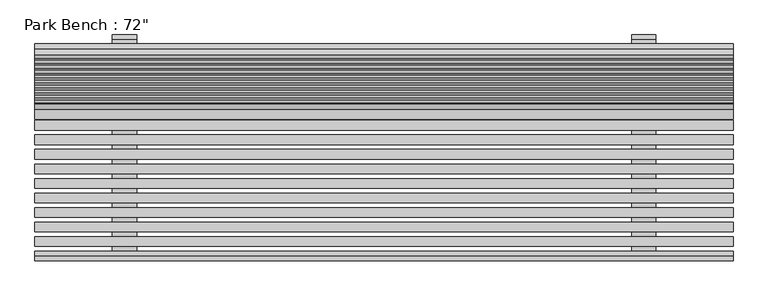
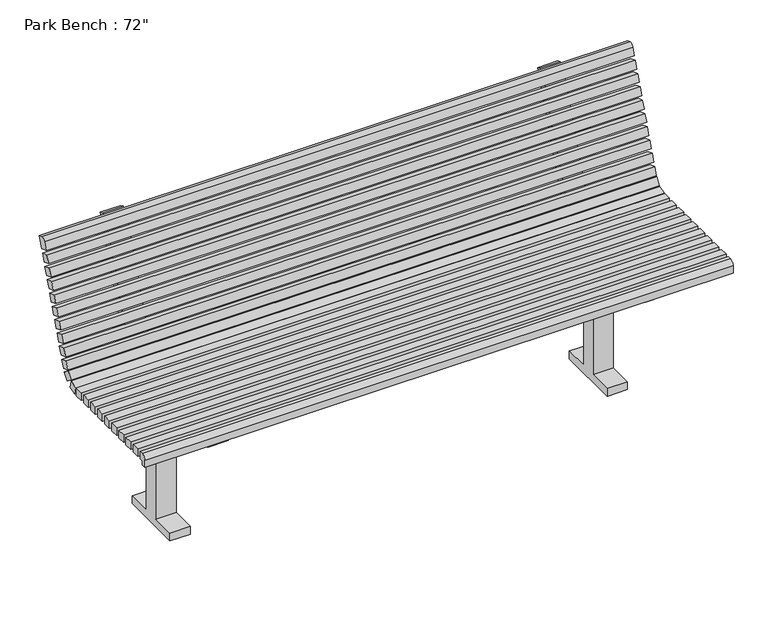
"""IFC4 building model written with IfcOpenShell, lengths in millimetres: geographic element geometry."""

from ifc_helpers import new_model, si_unit, point, frame, frame_2d, origin, place, context, project, spatial, polyline, circle_curve, trimmed, segment, composite_curve, outline, extrude, source, transform, mapped, element, save


def geographic_element_235d1464(model_context):
    return source(origin(), model_context, "Body", "SweptSolid", [
        extrude(outline(polyline([(914.4, -255.4337104), (914.4, -280.8337104), (-914.4, -280.8337104), (-914.4, -255.4337104), (914.4, -255.4337104)])), frame((0.0, 0.0, 457.2), z_axis=(0.0, 0.0, 1.0), x_axis=(1.0, 0.0, 0.0)), (0.0, 0.0, 1.0), 25.4),
        extrude(outline(polyline([(914.4, -217.3337104), (914.4, -242.7337104), (-914.4, -242.7337104), (-914.4, -217.3337104), (914.4, -217.3337104)])), frame((0.0, 0.0, 457.2), z_axis=(0.0, 0.0, 1.0), x_axis=(1.0, 0.0, 0.0)), (0.0, 0.0, 1.0), 25.4),
        extrude(outline(polyline([(914.4, -179.2337104), (914.4, -204.6337104), (-914.4, -204.6337104), (-914.4, -179.2337104), (914.4, -179.2337104)])), frame((0.0, 0.0, 457.2), z_axis=(0.0, 0.0, 1.0), x_axis=(1.0, 0.0, 0.0)), (0.0, 0.0, 1.0), 25.4),
        extrude(outline(polyline([(914.4, -141.1337104), (914.4, -166.5337104), (-914.4, -166.5337104), (-914.4, -141.1337104), (914.4, -141.1337104)])), frame((0.0, 0.0, 457.2), z_axis=(0.0, 0.0, 1.0), x_axis=(1.0, 0.0, 0.0)), (0.0, 0.0, 1.0), 25.4),
        extrude(outline(polyline([(914.4, -103.0337104), (914.4, -128.4337104), (-914.4, -128.4337104), (-914.4, -103.0337104), (914.4, -103.0337104)])), frame((0.0, 0.0, 457.2), z_axis=(0.0, 0.0, 1.0), x_axis=(1.0, 0.0, 0.0)), (0.0, 0.0, 1.0), 25.4),
        extrude(outline(polyline([(914.4, -64.9337104), (914.4, -90.3337104), (-914.4, -90.3337104), (-914.4, -64.9337104), (914.4, -64.9337104)])), frame((0.0, 0.0, 457.2), z_axis=(0.0, 0.0, 1.0), x_axis=(1.0, 0.0, 0.0)), (0.0, 0.0, 1.0), 25.4),
        extrude(outline(polyline([(914.4, -26.8337104), (914.4, -52.2337104), (-914.4, -52.2337104), (-914.4, -26.8337104), (914.4, -26.8337104)])), frame((0.0, 0.0, 457.2), z_axis=(0.0, 0.0, 1.0), x_axis=(1.0, 0.0, 0.0)), (0.0, 0.0, 1.0), 25.4),
        extrude(outline(polyline([(914.4, 11.2662896), (914.4, -14.1337104), (-914.4, -14.1337104), (-914.4, 11.2662896), (914.4, 11.2662896)])), frame((0.0, 0.0, 457.2), z_axis=(0.0, 0.0, 1.0), x_axis=(1.0, 0.0, 0.0)), (0.0, 0.0, 1.0), 25.4),
        extrude(outline(polyline([(914.4, 49.3662896), (914.4, 23.9662896), (-914.4, 23.9662896), (-914.4, 49.3662896), (914.4, 49.3662896)])), frame((0.0, 0.0, 457.2), z_axis=(0.0, 0.0, 1.0), x_axis=(1.0, 0.0, 0.0)), (0.0, 0.0, 1.0), 25.4),
        extrude(outline(composite_curve([segment(polyline([(-304.8, 457.2), (-304.8, 444.5), (-318.9337104, 444.5), (-318.9337104, 468.3125)]), True, "CONTINUOUS"), segment(trimmed(circle_curve(frame_2d((-304.6462104, 468.3125)), 14.2875), [point((-318.9337104, 468.3125))], [point((-304.6462104, 482.6))], False, "CARTESIAN"), True, "CONTINUOUS"), segment(polyline([(-304.6462104, 482.6), (-293.5337104, 482.6), (-293.5337104, 457.2), (-304.8, 457.2)]), True, "CONTINUOUS")], self_intersect=False)), frame((-914.4, 0.0, 0.0), z_axis=(1.0, 0.0, 0.0), x_axis=(0.0, 1.0, 0.0)), (0.0, 0.0, 1.0), 1828.8),
        extrude(outline(polyline([(0.0, -25.4), (0.0, 0.0), (1828.8, 0.0), (1828.8, -25.4), (0.0, -25.4)])), frame((914.4, 121.2738625, 585.5181247), z_axis=(0.0, 0.342020143325687, 0.9396926207859018), x_axis=(-1.0, 0.0, 0.0)), (0.0, 0.0, 1.0), 25.4),
        extrude(outline(polyline([(0.0, -25.4), (0.0, 0.0), (1828.8, 0.0), (1828.8, -25.4), (0.0, -25.4)])), frame((914.4, 134.30483, 621.3204136), z_axis=(0.0, 0.34202014332568254, 0.9396926207859034), x_axis=(-1.0, 0.0, 0.0)), (0.0, 0.0, 1.0), 25.4),
        extrude(outline(polyline([(0.0, -25.3999999), (0.0, 0.0), (1828.8, 0.0), (1828.8, -25.3999999), (0.0, -25.3999999)])), frame((914.4, 95.2119276, 513.913547), z_axis=(0.0, 0.34202014332568254, 0.9396926207859034), x_axis=(-1.0, 0.0, 0.0)), (0.0, 0.0, 1.0), 25.4),
        extrude(outline(polyline([(0.0, -25.4000001), (0.0, 0.0), (1828.8, 0.0), (1828.8, -25.4000001), (0.0, -25.4000001)])), frame((914.4, 108.242895, 549.7158359), z_axis=(0.0, 0.34202014332567804, 0.9396926207859051), x_axis=(-1.0, 0.0, 0.0)), (0.0, 0.0, 1.0), 25.4),
        extrude(outline(polyline([(0.0, -25.4), (0.0, 0.0), (1828.8, 0.0), (1828.8, -25.4), (0.0, -25.4)])), frame((914.4, 173.3977323, 728.7272801), z_axis=(0.0, 0.34202014332568337, 0.9396926207859031), x_axis=(-1.0, 0.0, 0.0)), (0.0, 0.0, 1.0), 25.4),
        extrude(outline(polyline([(0.0, -25.4000001), (0.0, 0.0), (1828.8, 0.0), (1828.8, -25.4000001), (0.0, -25.4000001)])), frame((914.4, 186.4286998, 764.529569), z_axis=(0.0, 0.3420201433256829, 0.9396926207859032), x_axis=(-1.0, 0.0, 0.0)), (0.0, 0.0, 1.0), 25.4),
        extrude(outline(polyline([(0.0, -25.4), (0.0, 0.0), (1828.8, 0.0), (1828.8, -25.4), (0.0, -25.4)])), frame((914.4, 147.3357974, 657.1227024), z_axis=(0.0, 0.3420201433256776, 0.9396926207859052), x_axis=(-1.0, 0.0, 0.0)), (0.0, 0.0, 1.0), 25.4),
        extrude(outline(polyline([(0.0, -25.4), (0.0, 0.0), (1828.8, 0.0), (1828.8, -25.4), (0.0, -25.4)])), frame((914.4, 160.3667649, 692.9249913), z_axis=(0.0, 0.34202014332568254, 0.9396926207859034), x_axis=(-1.0, 0.0, 0.0)), (0.0, 0.0, 1.0), 25.4),
        extrude(outline(polyline([(0.0, -25.3999999), (0.0, 0.0), (1828.8, 0.0), (1828.8, -25.3999999), (0.0, -25.3999999)])), frame((914.4, 199.4596673, 800.3318578), z_axis=(0.0, 0.3420201433256774, 0.9396926207859052), x_axis=(-1.0, 0.0, 0.0)), (0.0, 0.0, 1.0), 25.4),
        extrude(outline(composite_curve([segment(polyline([(249.3897948, 863.2491239), (236.3588273, 827.4468351), (212.4906347, 836.1341467), (221.1779464, 860.0023393)]), True, "CONTINUOUS"), segment(trimmed(circle_curve(frame_2d((233.1120426, 855.6586834)), 12.7), [point((221.1779464, 860.0023393))], [point((237.4556985, 867.5927797))], False, "CARTESIAN"), True, "CONTINUOUS"), segment(polyline([(237.4556985, 867.5927797), (249.3897948, 863.2491239)]), True, "CONTINUOUS")], self_intersect=False)), frame((-914.4, 0.0, 0.0), z_axis=(1.0, 0.0, 0.0), x_axis=(0.0, 1.0, 0.0)), (0.0, 0.0, 1.0), 1828.8),
        extrude(outline(polyline([(0.0, -25.4), (0.0, 0.0), (1828.8, 0.0), (1828.8, -25.4), (0.0, -25.4)])), frame((914.4, 78.7855779, 490.7267336), z_axis=(0.0, 0.5735764363510742, 0.8191520442889721), x_axis=(-1.0, 0.0, 0.0)), (0.0, 0.0, 1.0), 25.4),
        extrude(outline(polyline([(0.0, -25.4), (0.0, 0.0), (1828.8, 0.0), (1828.8, -25.4), (0.0, -25.4)])), frame((914.4, 59.0817015, 457.2297909), z_axis=(0.0, -0.2588190451024684, 0.9659258262890824), x_axis=(-1.0, 0.0, 0.0)), (0.0, 0.0, 1.0), 25.4),
        extrude(outline(composite_curve([segment(polyline([(-101.6, 25.4), (-25.4, 25.4), (-25.4, 431.8), (-304.8, 431.8), (-304.8, 457.2), (57.1368213, 457.2)]), True, "CONTINUOUS"), segment(trimmed(circle_curve(frame_2d((57.1368213, 520.7)), 63.5), [point((57.1368213, 457.2))], [point((116.8073027, 498.9817209))], True, "CARTESIAN"), True, "CONTINUOUS"), segment(polyline([(116.8073027, 498.9817209), (244.9406421, 851.0251774)]), True, "CONTINUOUS"), segment(trimmed(circle_curve(frame_2d((256.8747384, 846.6815216)), 12.7), [point((244.9406421, 851.0251774))], [point((261.2183942, 858.6156178))], False, "CARTESIAN"), True, "CONTINUOUS"), segment(polyline([(261.2183942, 858.6156178), (273.1524905, 854.271962), (140.6754953, 490.2944093)]), True, "CONTINUOUS"), segment(trimmed(circle_curve(frame_2d((57.1368213, 520.7)), 88.9), [point((140.6754953, 490.2944093))], [point((57.1368213, 431.8))], False, "CARTESIAN"), True, "CONTINUOUS"), segment(polyline([(57.1368213, 431.8), (25.4, 431.8), (25.4, 25.4), (101.6, 25.4), (101.6, 0.0), (-101.6, 0.0), (-101.6, 25.4)]), True, "CONTINUOUS")], self_intersect=False)), frame((648.3736591, 0.0, 0.0), z_axis=(1.0, 0.0, 0.0), x_axis=(0.0, 1.0, 0.0)), (0.0, 0.0, 1.0), 62.8263409),
        extrude(outline(composite_curve([segment(polyline([(-101.6, 25.4), (-25.4, 25.4), (-25.4, 431.8), (-304.8, 431.8), (-304.8, 457.2), (57.1368213, 457.2)]), True, "CONTINUOUS"), segment(trimmed(circle_curve(frame_2d((57.1368213, 520.7)), 63.5), [point((57.1368213, 457.2))], [point((116.8073027, 498.9817209))], True, "CARTESIAN"), True, "CONTINUOUS"), segment(polyline([(116.8073027, 498.9817209), (244.9406421, 851.0251774)]), True, "CONTINUOUS"), segment(trimmed(circle_curve(frame_2d((256.8747384, 846.6815216)), 12.7), [point((244.9406421, 851.0251774))], [point((261.2183942, 858.6156178))], False, "CARTESIAN"), True, "CONTINUOUS"), segment(polyline([(261.2183942, 858.6156178), (273.1524905, 854.271962), (140.6754953, 490.2944093)]), True, "CONTINUOUS"), segment(trimmed(circle_curve(frame_2d((57.1368213, 520.7)), 88.9), [point((140.6754953, 490.2944093))], [point((57.1368213, 431.8))], False, "CARTESIAN"), True, "CONTINUOUS"), segment(polyline([(57.1368213, 431.8), (25.4, 431.8), (25.4, 25.4), (101.6, 25.4), (101.6, 0.0), (-101.6, 0.0), (-101.6, 25.4)]), True, "CONTINUOUS")], self_intersect=False)), frame((-711.2, 0.0, 0.0), z_axis=(1.0, 0.0, 0.0), x_axis=(0.0, 1.0, 0.0)), (0.0, 0.0, 1.0), 63.8916859),
    ])


if __name__ == "__main__":
    model = new_model("IFC4")
    model_context = context("Model", 3, world=origin())
    ifc_project = project(units=[si_unit("LENGTHUNIT", "METRE", prefix="MILLI")], contexts=[model_context])
    site = spatial("IfcSite", under=ifc_project)
    building = spatial("IfcBuilding", under=site)
    placement = place(None, origin())
    geographic_element_shape = geographic_element_235d1464(model_context)
    element("IfcGeographicElement", 1, ObjectType="Park Bench : 72\"", at=placement, inside=building, context=model_context, shape_type="MappedRepresentation", body=[
        mapped(geographic_element_shape, transform((0.0, 0.0, 0.0), x_axis=(1.0, 0.0, 0.0), y_axis=(0.0, 1.0, 0.0), z_axis=(0.0, 0.0, 1.0))),
    ])
    save(model, "model.ifc")

# Revit data of these elements
# Type "Park Bench : 72\""
#   Length = 6' - 0"
#   Seat Material = Wood - Teak
#   Frame Material = Steel, Paint Finish, Dark Gray, Matte
# Element 1 (IfcGeographicElement, "Park Bench : 72\"")
#   Materials on its faces: "Wood - Teak", "Steel, Paint Finish, Dark Gray, Matte"
# Materials
#   "Wood - Teak": class "Wood", colour RGB 145 112 90, transparency 0
#   "Steel, Paint Finish, Dark Gray, Matte": class "Metal", colour RGB 0 0 0, transparency 0, Description = "Steel, paint finish, dark gray, matte", Cost = 0
